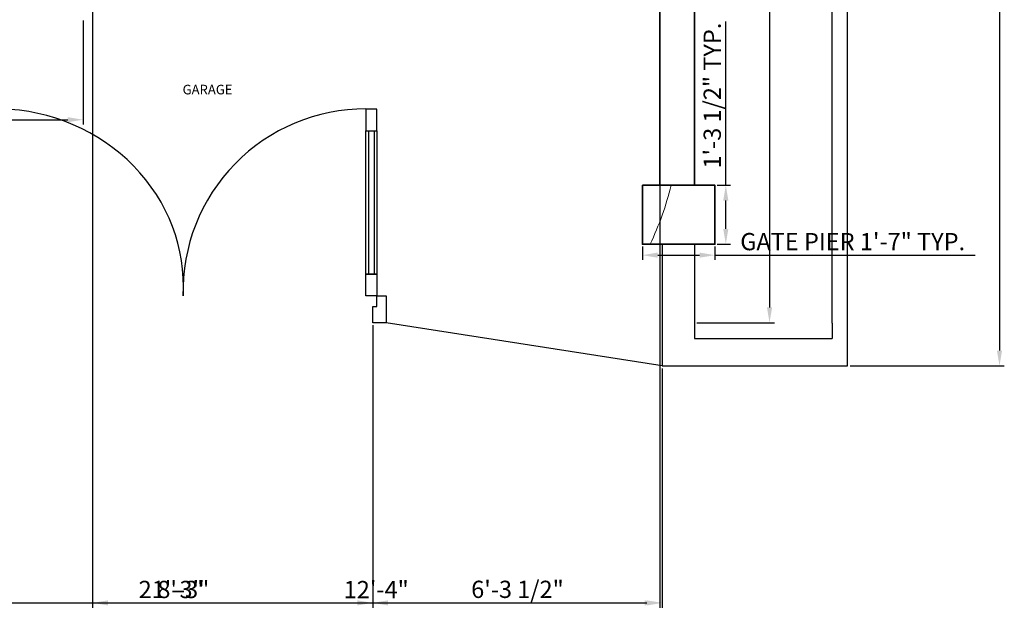
# Model space of a CAD drawing. Units: inches. Extents: x 1239 to 2276906, y 2273 to 321338.
# Tile 12 of 23: x 1754 to 2011, y 2273 to 2429. Entities that reach past the tile are written whole.
import ezdxf

# ---------------------------------------------------------------- set-up
doc = ezdxf.new("R2010")
doc.units = ezdxf.units.IN
for name, color, linetype, lineweight in [('A-ANNO-DIMS', 2, 'Continuous', 18), ('A-AREA-IDEN', 7, 'Continuous', 18), ('A-COLS', 7, 'Continuous', 35), ('C-PRKG', 8, 'Continuous', 13), ('C-PROP', 7, 'Continuous', 25), ('L-SITE-GATE', 1, 'Continuous', 25), ('wall', 7, 'Continuous', 35)]:
    doc.layers.add(name, color=color, linetype=linetype, lineweight=lineweight)
doc.styles.get("Standard").update_dxf_attribs({"font": 'arial.ttf'})
doc.dimstyles.new('ISO-25', dxfattribs={"dimtxt": 4.5, "dimasz": 4, "dimexe": 1.25, "dimexo": 0.625, "dimtad": 1, "dimdec": 1, "dimlunit": 3, "dimtxsty": 'Standard', "dimcen": 2.5, "dimadec": 0, "dimazin": 0, "dimtfac": 1, "dimtdec": 1, "dimtmove": 0, "dimatfit": 3, "dimfxl": 1, "dimarcsym": 0})

# ---------------------------------------------------------------- blocks, each defined once
blk = doc.blocks.new('*D38')
at = {"layer": 'A-ANNO-DIMS', "color": 0, "lineweight": -2, "transparency": 16777216}
for p, q in [((1971.01, 3545.9), (2011.25, 3545.9)), ((2010, 3541.9), (2010, 2342.75)), ((1971.01, 2338.75), (2011.25, 2338.75))]:
    blk.add_line(p, q, dxfattribs=at)
at = {"layer": 'A-ANNO-DIMS', "color": 0, "transparency": 16777216}
for points in [[(2009.33, 3541.9), (2010.67, 3541.9), (2010, 3545.9)], [(2009.33, 2342.75), (2010.67, 2342.75), (2010, 2338.75)]]:
    blk.add_solid(points, dxfattribs=at)
at = {"layer": 'Defpoints', "color": 0, "transparency": 16777216}
for p in [(1970.38, 3545.9), (1970.38, 2338.75), (2010, 2338.75)]:
    blk.add_point(p, dxfattribs=at)
at = {"layer": 'A-ANNO-DIMS', "color": 0, "transparency": 16777216, "insert": (2007.08, 2942.32), "char_height": 4.5, "attachment_point": 5, "rotation": 90}
blk.add_mtext('100\'-7.2"', dxfattribs=at)
blk = doc.blocks.new('*D40')
at = {"layer": 'A-ANNO-DIMS', "color": 0, "lineweight": -2, "transparency": 16777216}
for p, q in [((1931.01, 3505.9), (1951.25, 3505.9)), ((1950, 3501.9), (1950, 2354)), ((1931.01, 2350), (1951.25, 2350))]:
    blk.add_line(p, q, dxfattribs=at)
at = {"layer": 'A-ANNO-DIMS', "color": 0, "transparency": 16777216}
for points in [[(1949.33, 3501.9), (1950.67, 3501.9), (1950, 3505.9)], [(1949.33, 2354), (1950.67, 2354), (1950, 2350)]]:
    blk.add_solid(points, dxfattribs=at)
at = {"layer": 'Defpoints', "color": 0, "transparency": 16777216}
for p in [(1930.38, 3505.9), (1930.38, 2350), (1950, 2350)]:
    blk.add_point(p, dxfattribs=at)
at = {"layer": 'A-ANNO-DIMS', "color": 0, "transparency": 16777216, "insert": (1947.08, 2927.95), "char_height": 4.5, "attachment_point": 5, "rotation": 90}
blk.add_mtext('96\'-3.9"', dxfattribs=at)
blk = doc.blocks.new('SITE-PIER')
blk.add_lwpolyline([(0, 15.4), (18.94, 15.4), (18.94, 0), (0, 0)], close=True)
blk = doc.blocks.new('*D56')
at = {"layer": 'A-ANNO-DIMS', "color": 0, "lineweight": -2, "transparency": 16777216}
for p, q in [((1916.81, 2369.87), (1916.81, 2366.4)), ((1935.75, 2369.87), (1935.75, 2366.4)), ((1920.81, 2367.65), (1931.75, 2367.65)), ((1935.75, 2367.65), (2003.63, 2367.65))]:
    blk.add_line(p, q, dxfattribs=at)
at = {"layer": 'A-ANNO-DIMS', "color": 0, "transparency": 16777216}
for points in [[(1920.81, 2368.32), (1920.81, 2366.99), (1916.81, 2367.65)], [(1931.75, 2368.32), (1931.75, 2366.99), (1935.75, 2367.65)]]:
    blk.add_solid(points, dxfattribs=at)
at = {"layer": 'Defpoints', "color": 0, "transparency": 16777216}
for p in [(1916.81, 2370.49), (1935.75, 2370.49), (1935.75, 2367.65)]:
    blk.add_point(p, dxfattribs=at)
at = {"layer": 'A-ANNO-DIMS', "color": 0, "transparency": 16777216, "insert": (1971.69, 2370.6), "char_height": 4.5, "attachment_point": 5}
blk.add_mtext('GATE PIER 1\'-7" TYP.', dxfattribs=at)
blk = doc.blocks.new('*D57')
at = {"layer": 'A-ANNO-DIMS', "color": 0, "lineweight": -2, "transparency": 16777216}
for p, q in [((1938.59, 2385.9), (1938.59, 2428.64)), ((1936.37, 2385.9), (1939.84, 2385.9)), ((1938.59, 2374.49), (1938.59, 2381.9)), ((1936.37, 2370.49), (1939.84, 2370.49))]:
    blk.add_line(p, q, dxfattribs=at)
at = {"layer": 'A-ANNO-DIMS', "color": 0, "transparency": 16777216}
for points in [[(1937.92, 2381.9), (1939.25, 2381.9), (1938.59, 2385.9)], [(1937.92, 2374.49), (1939.25, 2374.49), (1938.59, 2370.49)]]:
    blk.add_solid(points, dxfattribs=at)
at = {"layer": 'Defpoints', "color": 0, "transparency": 16777216}
for p in [(1935.75, 2385.9), (1938.59, 2385.9), (1935.75, 2370.49)]:
    blk.add_point(p, dxfattribs=at)
at = {"layer": 'A-ANNO-DIMS', "color": 0, "transparency": 16777216, "insert": (1935.63, 2409.27), "char_height": 4.5, "attachment_point": 5, "rotation": 90}
blk.add_mtext('1\'-3 1/2" TYP.', dxfattribs=at)
blk = doc.blocks.new('*D59')
at = {"layer": 'A-ANNO-DIMS', "color": 0, "lineweight": -2, "transparency": 16777216}
for p, q in [((1701.8, 2428.88), (1701.8, 2401.73)), ((1770.89, 2428.88), (1770.89, 2401.73)), ((1705.8, 2402.98), (1766.89, 2402.98))]:
    blk.add_line(p, q, dxfattribs=at)
at = {"layer": 'A-ANNO-DIMS', "color": 0, "transparency": 16777216}
for points in [[(1705.8, 2403.65), (1705.8, 2402.31), (1701.8, 2402.98)], [(1766.89, 2403.65), (1766.89, 2402.31), (1770.89, 2402.98)]]:
    blk.add_solid(points, dxfattribs=at)
at = {"layer": 'Defpoints', "color": 0, "transparency": 16777216}
for p in [(1701.8, 2429.5), (1770.89, 2429.5), (1770.89, 2402.98)]:
    blk.add_point(p, dxfattribs=at)
at = {"layer": 'A-ANNO-DIMS', "color": 0, "transparency": 16777216, "insert": (1736.34, 2405.9), "char_height": 4.5, "attachment_point": 5}
blk.add_mtext('5\'-9" TYP.', dxfattribs=at)
blk = doc.blocks.new('*D87')
at = {"layer": 'A-ANNO-DIMS', "color": 0, "lineweight": -2, "transparency": 16777216}
for p, q in [((1666.38, 3250.77), (1666.38, 2275.7)), ((1921.38, 3250.77), (1921.38, 2275.7)), ((1670.38, 2276.95), (1917.38, 2276.95))]:
    blk.add_line(p, q, dxfattribs=at)
at = {"layer": 'A-ANNO-DIMS', "color": 0, "transparency": 16777216}
for points in [[(1670.38, 2277.61), (1670.38, 2276.28), (1666.38, 2276.95)], [(1917.38, 2277.61), (1917.38, 2276.28), (1921.38, 2276.95)]]:
    blk.add_solid(points, dxfattribs=at)
at = {"layer": 'Defpoints', "color": 0, "transparency": 16777216}
for p in [(1666.38, 3251.4), (1921.38, 3251.4), (1921.38, 2276.95)]:
    blk.add_point(p, dxfattribs=at)
at = {"layer": 'A-ANNO-DIMS', "color": 0, "transparency": 16777216, "insert": (1793.88, 2279.87), "char_height": 4.5, "attachment_point": 5}
blk.add_mtext('21\'-3"', dxfattribs=at)
blk = doc.blocks.new('*D99')
at = {"layer": 'A-ANNO-DIMS', "color": 0, "lineweight": -2, "transparency": 16777216}
for p, q in [((1773.38, 2854.77), (1773.38, 2275.7)), ((1921.38, 2854.77), (1921.38, 2275.7)), ((1777.38, 2276.95), (1917.38, 2276.95))]:
    blk.add_line(p, q, dxfattribs=at)
at = {"layer": 'A-ANNO-DIMS', "color": 0, "transparency": 16777216}
for points in [[(1777.38, 2277.61), (1777.38, 2276.28), (1773.38, 2276.95)], [(1917.38, 2277.61), (1917.38, 2276.28), (1921.38, 2276.95)]]:
    blk.add_solid(points, dxfattribs=at)
at = {"layer": 'Defpoints', "color": 0, "transparency": 16777216}
for p in [(1773.38, 2855.4), (1921.38, 2855.4), (1921.38, 2276.95)]:
    blk.add_point(p, dxfattribs=at)
at = {"layer": 'A-ANNO-DIMS', "color": 0, "transparency": 16777216, "insert": (1847.38, 2279.83), "char_height": 4.5, "attachment_point": 5}
blk.add_mtext('12\'-4"', dxfattribs=at)
blk = doc.blocks.new('*D101')
at = {"layer": 'A-ANNO-DIMS', "color": 0, "lineweight": -2, "transparency": 16777216}
for p, q in [((1747.63, 2349.38), (1747.63, 2275.7)), ((1846.47, 2349.38), (1846.47, 2275.7)), ((1751.63, 2276.95), (1842.47, 2276.95))]:
    blk.add_line(p, q, dxfattribs=at)
at = {"layer": 'A-ANNO-DIMS', "color": 0, "transparency": 16777216}
for points in [[(1751.63, 2277.61), (1751.63, 2276.28), (1747.63, 2276.95)], [(1842.47, 2277.61), (1842.47, 2276.28), (1846.47, 2276.95)]]:
    blk.add_solid(points, dxfattribs=at)
at = {"layer": 'Defpoints', "color": 0, "transparency": 16777216}
for p in [(1747.63, 2350), (1846.47, 2350), (1846.47, 2276.95)]:
    blk.add_point(p, dxfattribs=at)
at = {"layer": 'A-ANNO-DIMS', "color": 0, "transparency": 16777216, "insert": (1797.05, 2279.87), "char_height": 4.5, "attachment_point": 5}
blk.add_mtext('8\'-3"', dxfattribs=at)
blk = doc.blocks.new('*D113')
at = {"layer": 'A-ANNO-DIMS', "color": 0, "lineweight": -2, "transparency": 16777216}
for p, q in [((1846.47, 2349.38), (1846.47, 2275.7)), ((1922, 2338.12), (1922, 2275.7)), ((1850.47, 2276.95), (1918, 2276.95))]:
    blk.add_line(p, q, dxfattribs=at)
at = {"layer": 'A-ANNO-DIMS', "color": 0, "transparency": 16777216}
for points in [[(1850.47, 2277.61), (1850.47, 2276.28), (1846.47, 2276.95)], [(1918, 2277.61), (1918, 2276.28), (1922, 2276.95)]]:
    blk.add_solid(points, dxfattribs=at)
at = {"layer": 'Defpoints', "color": 0, "transparency": 16777216}
for p in [(1846.47, 2350), (1922, 2338.75), (1922, 2276.95)]:
    blk.add_point(p, dxfattribs=at)
at = {"layer": 'A-ANNO-DIMS', "color": 0, "transparency": 16777216, "insert": (1884.23, 2279.9), "char_height": 4.5, "attachment_point": 5}
blk.add_mtext('6\'-3 1/2"', dxfattribs=at)

msp = doc.modelspace()

# ---------------------------------------------------------------- linework, layer by layer
at = {"layer": 'C-PRKG'}
msp.add_arc((1851.04, 2403.31), 75.3, 334.1615, 346.6284, dxfattribs=at)
at = {"layer": 'C-PROP'}
for p, q in [((1922, 2370.49), (1922, 2366.49)), ((1930.38, 2370.49), (1930.38, 2345.9)), ((1922, 2366.49), (1922, 2338.75)), ((1922, 2338.75), (1850, 2350)), ((1966.38, 2349.9), (1966.38, 2345.9)), ((1930.38, 2345.9), (1966.38, 2345.9)), ((1970.38, 2338.75), (1970.38, 2345.9)), ((1922, 2338.75), (1970.38, 2338.75))]:
    msp.add_line(p, q, dxfattribs=at)
for points in [[(1970.38, 2345.9), (1970.38, 3545.9), (1310.38, 3545.9), (1310.38, 2345.9), (1644.79, 2345.9)], [(1966.38, 2349.9), (1966.38, 3541.9), (1314.38, 3541.9), (1314.38, 2607.52)]]:
    msp.add_lwpolyline(points, dxfattribs=at)
at = {"layer": 'L-SITE-GATE'}
for p, q in [((1844.71, 2405.77), (1844.71, 2400.12)), ((1847.53, 2405.77), (1844.71, 2405.77)), ((1847.53, 2400.12), (1847.53, 2405.77)), ((1844.71, 2400.12), (1847.53, 2400.12)), ((1844.71, 2362.71), (1844.71, 2400.12)), ((1844.71, 2400.12), (1847.53, 2400.12)), ((1845.41, 2362.71), (1845.41, 2400.12)), ((1845.41, 2400.12), (1846.82, 2400.12)), ((1846.82, 2400.12), (1846.82, 2362.71)), ((1847.53, 2400.12), (1847.53, 2362.71)), ((1847.53, 2362.71), (1844.71, 2362.71)), ((1844.71, 2357.06), (1844.71, 2362.71)), ((1844.71, 2362.71), (1847.53, 2362.71)), ((1846.82, 2362.71), (1845.41, 2362.71)), ((1847.53, 2362.71), (1847.53, 2357.06)), ((1847.53, 2357.06), (1844.71, 2357.06)), ((1847.53, 2357.06), (1850, 2357.06)), ((1847.53, 2354.24), (1847.53, 2357.06)), ((1850, 2357.06), (1850, 2350)), ((1846.47, 2353.53), (1846.47, 2354.24)), ((1846.47, 2354.24), (1847.53, 2354.24)), ((1846.47, 2350), (1846.47, 2353.53)), ((1850, 2350), (1846.47, 2350))]:
    msp.add_line(p, q, dxfattribs=at)
msp.add_arc((1844.51, 2358.26), 47.52, 89.7657, 181.4438, dxfattribs=at)
msp.add_ellipse((1749.32, 2360.67), major_axis=(47.08, -8.59), ratio=0.940794, start_param=0.11153, end_param=1.73917, dxfattribs=at)
at = {"layer": 'wall'}
for p, q in [((1930.38, 2385.9), (1930.38, 3505.9)), ((1921.38, 2394.9), (1921.38, 2942.4)), ((1921.38, 2394.9), (1921.38, 2385.9)), ((1921.38, 2385.9), (1930.38, 2385.9))]:
    msp.add_line(p, q, dxfattribs=at)

# ---------------------------------------------------------------- block references
at = {"layer": 'A-COLS'}
msp.add_blockref('SITE-PIER', (1916.81, 2370.49), dxfattribs=at)

# ---------------------------------------------------------------- texts
at = {"layer": 'A-AREA-IDEN', "insert": (1796.86, 2412.09), "char_height": 2.5, "attachment_point": 1}
msp.add_mtext_dynamic_manual_height_columns('GARAGE', width=44.9462, gutter_width=12.5, heights=[0], dxfattribs=at)

# ---------------------------------------------------------------- dimensions: what is measured, and where the dimension line sits
at = {"layer": 'A-ANNO-DIMS'}
for base, p1, p2, picture, middle in [((2010, 2338.7461), (1970.3833, 3545.8972), (1970.3833, 2338.7461), '*D38', (2007.0774, 2942.3216)), ((1950, 2350), (1930.38, 3505.9), (1930.38, 2350), '*D40', (1947.08, 2927.95))]:
    dim = msp.add_linear_dim(base=base, p1=p1, p2=p2, angle=90, dimstyle='ISO-25', override={"dimclrd": 0, "dimclre": 0, "dimclrt": 0}, dxfattribs=at)
    dim.commit()
    dim.dimension.update_dxf_attribs({"geometry": picture, "text_midpoint": middle})
for base, p1, p2, picture, middle in [((1921.38, 2276.95), (1666.38, 3251.4), (1921.38, 3251.4), '*D87', (1793.88, 2279.87)), ((1921.38, 2276.95), (1773.38, 2855.4), (1921.38, 2855.4), '*D99', (1847.38, 2279.83)), ((1846.47, 2276.95), (1747.63, 2350), (1846.47, 2350), '*D101', (1797.05, 2279.87)), ((1922, 2276.95), (1846.47, 2350), (1922, 2338.75), '*D113', (1884.23, 2279.9))]:
    dim = msp.add_linear_dim(base=base, p1=p1, p2=p2, dimstyle='ISO-25', override={"dimdec": 1, "dimlfac": 1, "dimrnd": 0, "dimzin": 1, "dimdsep": 46, "dimlunit": 4, "dimfrac": 2}, dxfattribs=at)
    dim.commit()
    dim.dimension.update_dxf_attribs({"geometry": picture, "text_midpoint": middle})
for base, p1, p2, angle, picture, middle in [((1770.89, 2402.98), (1701.8, 2429.5), (1770.89, 2429.5), 360, '*D59', (1736.34, 2405.9)), ((1938.59, 2385.9), (1935.75, 2370.49), (1935.75, 2385.9), 90, '*D57', (1935.63, 2409.27))]:
    dim = msp.add_linear_dim(base=base, p1=p1, p2=p2, angle=angle, text='<> TYP.', dimstyle='ISO-25', override={"dimdec": 1, "dimlfac": 1, "dimrnd": 0, "dimzin": 1, "dimdsep": 46, "dimlunit": 4, "dimfrac": 2}, dxfattribs=at)
    dim.commit()
    dim.dimension.update_dxf_attribs({"geometry": picture, "text_midpoint": middle})
dim = msp.add_linear_dim(base=(1935.75, 2367.65), p1=(1916.81, 2370.49), p2=(1935.75, 2370.49), text='GATE PIER <> TYP.', dimstyle='ISO-25', override={"dimdec": 1, "dimlfac": 1, "dimrnd": 0, "dimzin": 1, "dimdsep": 46, "dimlunit": 4, "dimfrac": 2}, dxfattribs=at)
dim.commit()
dim.dimension.update_dxf_attribs({"geometry": '*D56', "text_midpoint": (1971.69, 2370.6)})

doc.saveas('drawing.dxf')
